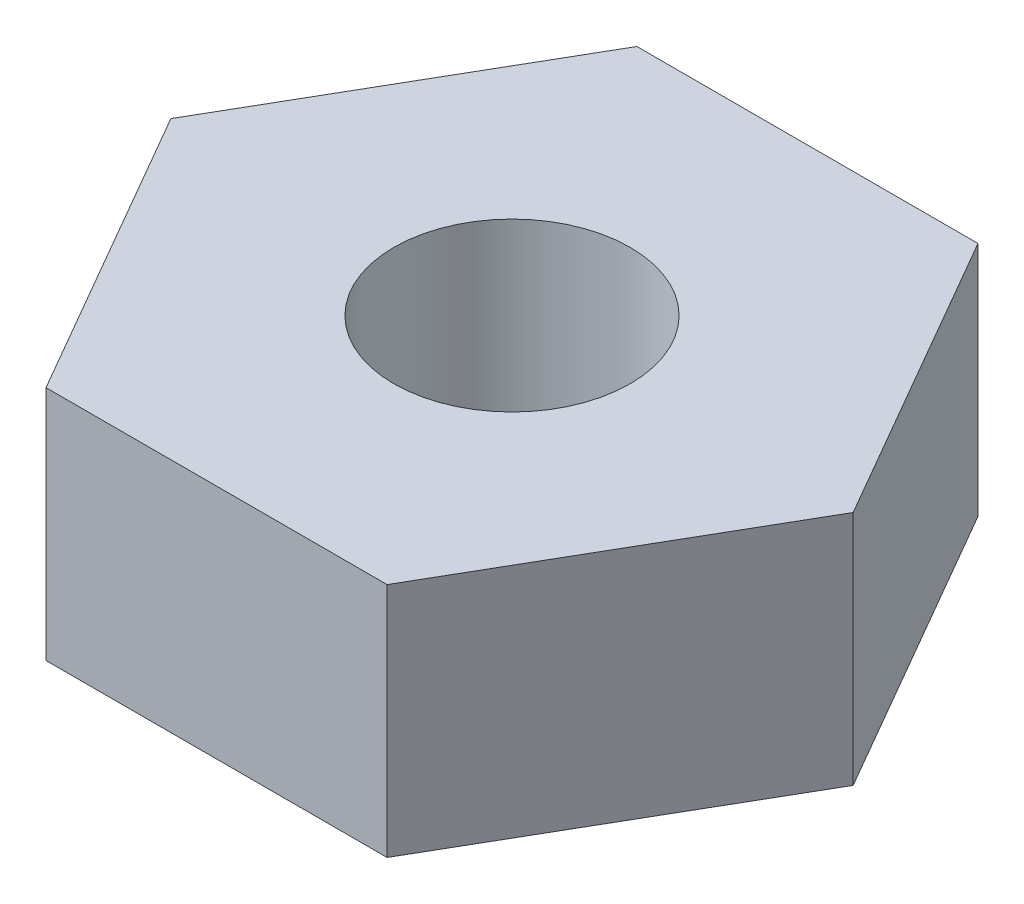
ISO-10303-21;
HEADER;
FILE_DESCRIPTION(('STEP AP214'),'2;1');
FILE_NAME('part.step','',(''),(''),'','','');
FILE_SCHEMA(('AUTOMOTIVE_DESIGN { 1 0 10303 214 1 1 1 1 }'));
ENDSEC;
DATA;
#1=APPLICATION_CONTEXT('core data for automotive mechanical design processes');
#2=APPLICATION_PROTOCOL_DEFINITION('international standard','automotive_design',2000,#1);
#3=PRODUCT_CONTEXT('',#1,'mechanical');
#4=PRODUCT('Part','Part','',(#3));
#5=PRODUCT_RELATED_PRODUCT_CATEGORY('part','',(#4));
#6=PRODUCT_DEFINITION_FORMATION('','',#4);
#7=PRODUCT_DEFINITION_CONTEXT('part definition',#1,'design');
#8=PRODUCT_DEFINITION('design','',#6,#7);
#9=PRODUCT_DEFINITION_SHAPE('','',#8);
#10=(LENGTH_UNIT() NAMED_UNIT(*) SI_UNIT(.MILLI.,.METRE.));
#11=(NAMED_UNIT(*) PLANE_ANGLE_UNIT() SI_UNIT($,.RADIAN.));
#12=(NAMED_UNIT(*) SI_UNIT($,.STERADIAN.) SOLID_ANGLE_UNIT());
#13=UNCERTAINTY_MEASURE_WITH_UNIT(LENGTH_MEASURE(1.E-05),#10,'distance_accuracy_value','');
#14=(GEOMETRIC_REPRESENTATION_CONTEXT(3) GLOBAL_UNCERTAINTY_ASSIGNED_CONTEXT((#13)) GLOBAL_UNIT_ASSIGNED_CONTEXT((#10,
#11,#12)) REPRESENTATION_CONTEXT('',''));
#15=CARTESIAN_POINT('',(0.,0.,0.));
#16=DIRECTION('',(0.,0.,1.));
#17=DIRECTION('',(1.,0.,0.));
#18=AXIS2_PLACEMENT_3D('',#15,#16,#17);
#19=CARTESIAN_POINT('',(0.,10.,0.));
#20=DIRECTION('',(0.,1.,0.));
#21=DIRECTION('',(0.,0.,1.));
#22=AXIS2_PLACEMENT_3D('',#19,#20,#21);
#23=PLANE('',#22);
#24=DIRECTION('',(0.499999999999995,0.,-0.866025403784442));
#25=VECTOR('',#24,1.);
#26=CARTESIAN_POINT('',(14.4337567297409,10.,24.9999999999998));
#27=LINE('',#26,#25);
#28=CARTESIAN_POINT('',(14.4337567297409,10.,24.9999999999998));
#29=VERTEX_POINT('',#28);
#30=CARTESIAN_POINT('',(28.8675134594813,10.,0.));
#31=VERTEX_POINT('',#30);
#32=EDGE_CURVE('E132',#29,#31,#27,.T.);
#33=ORIENTED_EDGE('',*,*,#32,.T.);
#34=DIRECTION('',(-0.500000000000001,0.,-0.866025403784438));
#35=VECTOR('',#34,1.);
#36=CARTESIAN_POINT('',(28.8675134594813,10.,0.));
#37=LINE('',#36,#35);
#38=CARTESIAN_POINT('',(14.4337567297406,10.,-25.));
#39=VERTEX_POINT('',#38);
#40=EDGE_CURVE('E91',#31,#39,#37,.T.);
#41=ORIENTED_EDGE('',*,*,#40,.T.);
#42=DIRECTION('',(-1.,0.,0.));
#43=VECTOR('',#42,1.);
#44=CARTESIAN_POINT('',(14.4337567297406,10.,-25.));
#45=LINE('',#44,#43);
#46=CARTESIAN_POINT('',(-14.4337567297408,10.,-24.9999999999999));
#47=VERTEX_POINT('',#46);
#48=EDGE_CURVE('E106',#39,#47,#45,.T.);
#49=ORIENTED_EDGE('',*,*,#48,.T.);
#50=DIRECTION('',(-0.499999999999995,0.,0.866025403784441));
#51=VECTOR('',#50,1.);
#52=CARTESIAN_POINT('',(-14.4337567297408,10.,-24.9999999999999));
#53=LINE('',#52,#51);
#54=CARTESIAN_POINT('',(-28.8675134594813,10.,2.01580769085164E-13));
#55=VERTEX_POINT('',#54);
#56=EDGE_CURVE('E99',#47,#55,#53,.T.);
#57=ORIENTED_EDGE('',*,*,#56,.T.);
#58=DIRECTION('',(0.500000000000007,0.,0.866025403784435));
#59=VECTOR('',#58,1.);
#60=CARTESIAN_POINT('',(-28.8675134594813,10.,2.01580769085164E-13));
#61=LINE('',#60,#59);
#62=CARTESIAN_POINT('',(-14.4337567297404,10.,25.0000000000001));
#63=VERTEX_POINT('',#62);
#64=EDGE_CURVE('E102',#55,#63,#61,.T.);
#65=ORIENTED_EDGE('',*,*,#64,.T.);
#66=DIRECTION('',(1.,0.,0.));
#67=VECTOR('',#66,1.);
#68=CARTESIAN_POINT('',(-14.4337567297404,10.,25.0000000000001));
#69=LINE('',#68,#67);
#70=EDGE_CURVE('E57',#63,#29,#69,.T.);
#71=ORIENTED_EDGE('',*,*,#70,.T.);
#72=EDGE_LOOP('',(#33,#41,#49,#57,#65,#71));
#73=FACE_BOUND('',#72,.T.);
#74=CARTESIAN_POINT('',(0.,10.,0.));
#75=DIRECTION('',(0.,1.,0.));
#76=DIRECTION('',(0.,0.,1.));
#77=AXIS2_PLACEMENT_3D('',#74,#75,#76);
#78=CIRCLE('',#77,10.);
#79=CARTESIAN_POINT('',(0.,10.,10.));
#80=VERTEX_POINT('',#79);
#81=EDGE_CURVE('E126',#80,#80,#78,.T.);
#82=ORIENTED_EDGE('',*,*,#81,.F.);
#83=EDGE_LOOP('',(#82));
#84=FACE_BOUND('',#83,.T.);
#85=ADVANCED_FACE('F39',(#73,#84),#23,.T.);
#86=CARTESIAN_POINT('',(0.,-10.,0.));
#87=DIRECTION('',(0.,1.,0.));
#88=DIRECTION('',(0.,0.,1.));
#89=AXIS2_PLACEMENT_3D('',#86,#87,#88);
#90=PLANE('',#89);
#91=DIRECTION('',(0.499999999999995,0.,-0.866025403784442));
#92=VECTOR('',#91,1.);
#93=CARTESIAN_POINT('',(14.4337567297409,-10.,24.9999999999998));
#94=LINE('',#93,#92);
#95=CARTESIAN_POINT('',(14.4337567297409,-10.,24.9999999999998));
#96=VERTEX_POINT('',#95);
#97=CARTESIAN_POINT('',(28.8675134594813,-10.,0.));
#98=VERTEX_POINT('',#97);
#99=EDGE_CURVE('E122',#96,#98,#94,.T.);
#100=ORIENTED_EDGE('',*,*,#99,.F.);
#101=DIRECTION('',(1.,0.,0.));
#102=VECTOR('',#101,1.);
#103=CARTESIAN_POINT('',(-14.4337567297404,-10.,25.0000000000001));
#104=LINE('',#103,#102);
#105=CARTESIAN_POINT('',(-14.4337567297404,-10.,25.0000000000001));
#106=VERTEX_POINT('',#105);
#107=EDGE_CURVE('E84',#106,#96,#104,.T.);
#108=ORIENTED_EDGE('',*,*,#107,.F.);
#109=DIRECTION('',(0.500000000000007,0.,0.866025403784435));
#110=VECTOR('',#109,1.);
#111=CARTESIAN_POINT('',(-28.8675134594813,-10.,2.01580769085164E-13));
#112=LINE('',#111,#110);
#113=CARTESIAN_POINT('',(-28.8675134594813,-10.,2.01580769085164E-13));
#114=VERTEX_POINT('',#113);
#115=EDGE_CURVE('E79',#114,#106,#112,.T.);
#116=ORIENTED_EDGE('',*,*,#115,.F.);
#117=DIRECTION('',(-0.499999999999995,0.,0.866025403784441));
#118=VECTOR('',#117,1.);
#119=CARTESIAN_POINT('',(-14.4337567297408,-10.,-24.9999999999999));
#120=LINE('',#119,#118);
#121=CARTESIAN_POINT('',(-14.4337567297408,-10.,-24.9999999999999));
#122=VERTEX_POINT('',#121);
#123=EDGE_CURVE('E111',#122,#114,#120,.T.);
#124=ORIENTED_EDGE('',*,*,#123,.F.);
#125=DIRECTION('',(-1.,0.,0.));
#126=VECTOR('',#125,1.);
#127=CARTESIAN_POINT('',(14.4337567297406,-10.,-25.));
#128=LINE('',#127,#126);
#129=CARTESIAN_POINT('',(14.4337567297406,-10.,-25.));
#130=VERTEX_POINT('',#129);
#131=EDGE_CURVE('E128',#130,#122,#128,.T.);
#132=ORIENTED_EDGE('',*,*,#131,.F.);
#133=DIRECTION('',(-0.500000000000001,0.,-0.866025403784438));
#134=VECTOR('',#133,1.);
#135=CARTESIAN_POINT('',(28.8675134594813,-10.,0.));
#136=LINE('',#135,#134);
#137=EDGE_CURVE('E130',#98,#130,#136,.T.);
#138=ORIENTED_EDGE('',*,*,#137,.F.);
#139=EDGE_LOOP('',(#100,#108,#116,#124,#132,#138));
#140=FACE_BOUND('',#139,.T.);
#141=CARTESIAN_POINT('',(0.,-10.,0.));
#142=DIRECTION('',(0.,1.,0.));
#143=DIRECTION('',(0.,0.,1.));
#144=AXIS2_PLACEMENT_3D('',#141,#142,#143);
#145=CIRCLE('',#144,10.);
#146=CARTESIAN_POINT('',(0.,-10.,10.));
#147=VERTEX_POINT('',#146);
#148=EDGE_CURVE('E226',#147,#147,#145,.T.);
#149=ORIENTED_EDGE('',*,*,#148,.T.);
#150=EDGE_LOOP('',(#149));
#151=FACE_BOUND('',#150,.T.);
#152=ADVANCED_FACE('F145',(#140,#151),#90,.F.);
#153=CARTESIAN_POINT('',(14.4337567297409,10.,24.9999999999998));
#154=DIRECTION('',(-0.866025403784442,0.,-0.499999999999995));
#155=DIRECTION('',(-0.499999999999995,0.,0.866025403784442));
#156=AXIS2_PLACEMENT_3D('',#153,#154,#155);
#157=PLANE('',#156);
#158=ORIENTED_EDGE('',*,*,#99,.T.);
#159=DIRECTION('',(0.,-1.,0.));
#160=VECTOR('',#159,1.);
#161=CARTESIAN_POINT('',(28.8675134594813,10.,0.));
#162=LINE('',#161,#160);
#163=EDGE_CURVE('E11',#31,#98,#162,.T.);
#164=ORIENTED_EDGE('',*,*,#163,.F.);
#165=ORIENTED_EDGE('',*,*,#32,.F.);
#166=DIRECTION('',(0.,-1.,0.));
#167=VECTOR('',#166,1.);
#168=CARTESIAN_POINT('',(14.4337567297409,10.,24.9999999999998));
#169=LINE('',#168,#167);
#170=EDGE_CURVE('E117',#29,#96,#169,.T.);
#171=ORIENTED_EDGE('',*,*,#170,.T.);
#172=EDGE_LOOP('',(#158,#164,#165,#171));
#173=FACE_BOUND('',#172,.T.);
#174=ADVANCED_FACE('F41',(#173),#157,.F.);
#175=CARTESIAN_POINT('',(28.8675134594813,10.,0.));
#176=DIRECTION('',(-0.866025403784438,0.,0.500000000000001));
#177=DIRECTION('',(0.500000000000001,0.,0.866025403784438));
#178=AXIS2_PLACEMENT_3D('',#175,#176,#177);
#179=PLANE('',#178);
#180=ORIENTED_EDGE('',*,*,#137,.T.);
#181=DIRECTION('',(0.,-1.,0.));
#182=VECTOR('',#181,1.);
#183=CARTESIAN_POINT('',(14.4337567297406,10.,-25.));
#184=LINE('',#183,#182);
#185=EDGE_CURVE('E48',#39,#130,#184,.T.);
#186=ORIENTED_EDGE('',*,*,#185,.F.);
#187=ORIENTED_EDGE('',*,*,#40,.F.);
#188=ORIENTED_EDGE('',*,*,#163,.T.);
#189=EDGE_LOOP('',(#180,#186,#187,#188));
#190=FACE_BOUND('',#189,.T.);
#191=ADVANCED_FACE('F166',(#190),#179,.F.);
#192=CARTESIAN_POINT('',(14.4337567297406,10.,-25.));
#193=DIRECTION('',(0.,0.,1.));
#194=DIRECTION('',(1.,0.,0.));
#195=AXIS2_PLACEMENT_3D('',#192,#193,#194);
#196=PLANE('',#195);
#197=ORIENTED_EDGE('',*,*,#131,.T.);
#198=DIRECTION('',(0.,-1.,0.));
#199=VECTOR('',#198,1.);
#200=CARTESIAN_POINT('',(-14.4337567297408,10.,-24.9999999999999));
#201=LINE('',#200,#199);
#202=EDGE_CURVE('E113',#47,#122,#201,.T.);
#203=ORIENTED_EDGE('',*,*,#202,.F.);
#204=ORIENTED_EDGE('',*,*,#48,.F.);
#205=ORIENTED_EDGE('',*,*,#185,.T.);
#206=EDGE_LOOP('',(#197,#203,#204,#205));
#207=FACE_BOUND('',#206,.T.);
#208=ADVANCED_FACE('F143',(#207),#196,.F.);
#209=CARTESIAN_POINT('',(-14.4337567297408,10.,-24.9999999999999));
#210=DIRECTION('',(0.866025403784442,0.,0.499999999999995));
#211=DIRECTION('',(0.499999999999995,0.,-0.866025403784442));
#212=AXIS2_PLACEMENT_3D('',#209,#210,#211);
#213=PLANE('',#212);
#214=ORIENTED_EDGE('',*,*,#123,.T.);
#215=DIRECTION('',(0.,-1.,0.));
#216=VECTOR('',#215,1.);
#217=CARTESIAN_POINT('',(-28.8675134594813,10.,2.01580769085164E-13));
#218=LINE('',#217,#216);
#219=EDGE_CURVE('E112',#55,#114,#218,.T.);
#220=ORIENTED_EDGE('',*,*,#219,.F.);
#221=ORIENTED_EDGE('',*,*,#56,.F.);
#222=ORIENTED_EDGE('',*,*,#202,.T.);
#223=EDGE_LOOP('',(#214,#220,#221,#222));
#224=FACE_BOUND('',#223,.T.);
#225=ADVANCED_FACE('F115',(#224),#213,.F.);
#226=CARTESIAN_POINT('',(-28.8675134594813,10.,2.01580769085164E-13));
#227=DIRECTION('',(0.866025403784435,0.,-0.500000000000007));
#228=DIRECTION('',(-0.500000000000007,0.,-0.866025403784435));
#229=AXIS2_PLACEMENT_3D('',#226,#227,#228);
#230=PLANE('',#229);
#231=ORIENTED_EDGE('',*,*,#115,.T.);
#232=DIRECTION('',(0.,-1.,0.));
#233=VECTOR('',#232,1.);
#234=CARTESIAN_POINT('',(-14.4337567297404,10.,25.0000000000001));
#235=LINE('',#234,#233);
#236=EDGE_CURVE('E118',#63,#106,#235,.T.);
#237=ORIENTED_EDGE('',*,*,#236,.F.);
#238=ORIENTED_EDGE('',*,*,#64,.F.);
#239=ORIENTED_EDGE('',*,*,#219,.T.);
#240=EDGE_LOOP('',(#231,#237,#238,#239));
#241=FACE_BOUND('',#240,.T.);
#242=ADVANCED_FACE('F116',(#241),#230,.F.);
#243=CARTESIAN_POINT('',(-14.4337567297404,10.,25.0000000000001));
#244=DIRECTION('',(0.,0.,-1.));
#245=DIRECTION('',(-1.,0.,0.));
#246=AXIS2_PLACEMENT_3D('',#243,#244,#245);
#247=PLANE('',#246);
#248=ORIENTED_EDGE('',*,*,#107,.T.);
#249=ORIENTED_EDGE('',*,*,#170,.F.);
#250=ORIENTED_EDGE('',*,*,#70,.F.);
#251=ORIENTED_EDGE('',*,*,#236,.T.);
#252=EDGE_LOOP('',(#248,#249,#250,#251));
#253=FACE_BOUND('',#252,.T.);
#254=ADVANCED_FACE('F149',(#253),#247,.F.);
#255=CARTESIAN_POINT('',(0.,10.,0.));
#256=DIRECTION('',(0.,-1.,0.));
#257=DIRECTION('',(0.,0.,-1.));
#258=AXIS2_PLACEMENT_3D('',#255,#256,#257);
#259=CYLINDRICAL_SURFACE('',#258,10.);
#260=ORIENTED_EDGE('',*,*,#81,.T.);
#261=EDGE_LOOP('',(#260));
#262=FACE_BOUND('',#261,.T.);
#263=ORIENTED_EDGE('',*,*,#148,.F.);
#264=EDGE_LOOP('',(#263));
#265=FACE_BOUND('',#264,.T.);
#266=ADVANCED_FACE('F151',(#262,#265),#259,.F.);
#267=CLOSED_SHELL('',(#85,#152,#174,#191,#208,#225,#242,#254,#266));
#268=MANIFOLD_SOLID_BREP('B2',#267);
#269=ADVANCED_BREP_SHAPE_REPRESENTATION('',(#18,#268),#14);
#270=SHAPE_DEFINITION_REPRESENTATION(#9,#269);
ENDSEC;
END-ISO-10303-21;
